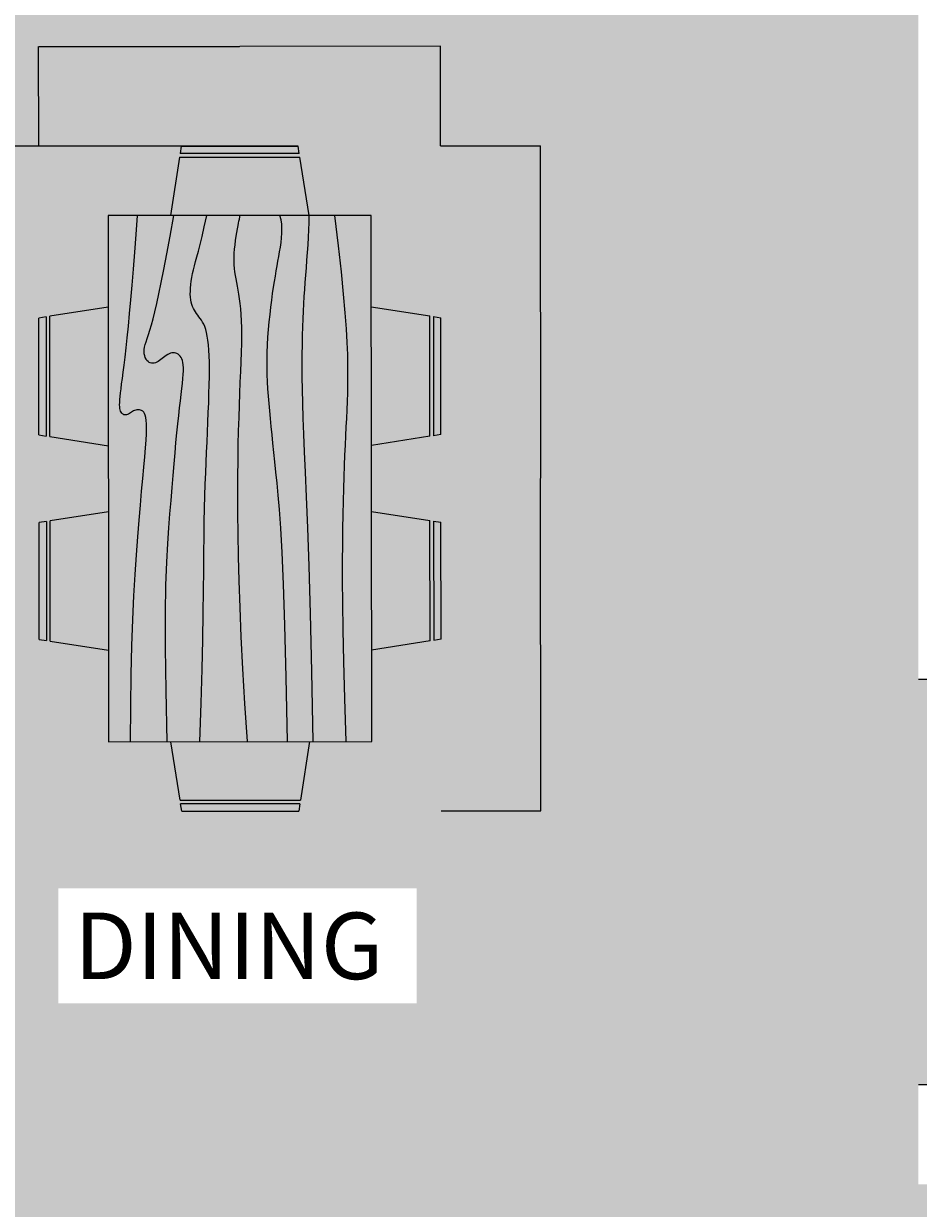
# Model space of a CAD drawing. Units: millimetres. Extents: x -229 to 16545, y -10488 to 4272.
# Tile 11 of 29: x 7347 to 9556, y -1268 to 1656. Entities that reach past the tile are written whole.
import ezdxf

# ---------------------------------------------------------------- set-up
doc = ezdxf.new("R2010")
doc.units = ezdxf.units.MM
for name, color, linetype, lineweight in [('A-ANNO-DIMS', 2, 'Continuous', 18), ('A-AREA-IDEN', 7, 'Continuous', 18), ('A-FURN', 8, 'Continuous', 18), ('A-FURN-PATT', 252, 'Continuous', 13)]:
    doc.layers.add(name, color=color, linetype=linetype, lineweight=lineweight)
doc.layers.add('A-FLOR-PATT', color=254, linetype='Continuous', lineweight=13, true_color=0xfeeab9)
doc.styles.get("Standard").update_dxf_attribs({"font": 'arial.ttf'})
doc.dimstyles.get("Standard").update_dxf_attribs({"dimtxt": 0.18, "dimasz": 0.18, "dimexe": 0.18, "dimexo": 0.0625, "dimgap": 0.09, "dimtad": 0, "dimtih": 1, "dimtoh": 1, "dimdec": 4, "dimzin": 0, "dimdsep": 46, "dimtxsty": 'Standard', "dimcen": 0.09, "dimadec": 0, "dimazin": 0, "dimtfac": 1, "dimtdec": 4, "dimtofl": 0, "dimtmove": 0, "dimatfit": 3, "dimfxl": 1, "dimtolj": 1, "dimtzin": 0, "dimarcsym": 0})

# ---------------------------------------------------------------- blocks, each defined once
blk = doc.blocks.new('Dining Set - 36 x 72 in.')
for p, q in [((-22.2343, 26.00059), (-23.4847, 17.99762)), ((-22.2304, 26), (-5.7608, 26)), ((-22, 27.5), (-22.1562, 26.50042)), ((-5.8416, 26.5), (-22.1534, 26.5)), ((-22, 27.5), (-6, 27.5)), ((-5.8437, 26.49966), (-6, 27.5)), ((-4.5152, 17.99762), (-5.7655, 25.99926)), ((5.7657, 26.00059), (4.5153, 17.99762)), ((5.7696, 26), (22.2392, 26)), ((6, 27.5), (5.8438, 26.50042)), ((22.1584, 26.5), (5.8466, 26.5)), ((6, 27.5), (22, 27.5)), ((22.1563, 26.49966), (22, 27.5)), ((23.4848, 17.99762), (22.2345, 25.99926)), ((36, 18), (-36, 18)), ((-36, 18), (-36, -18)), ((36, -18), (36, 18)), ((-45.5, 8), (-44.5004, 8.15617)), ((-44.5, -8.15843), (-44.5, 8.15338)), ((-44.0006, 8.23428), (-35.9976, 9.48474)), ((-44, 8.23041), (-44, -8.23915)), ((44.0006, 8.23428), (35.9976, 9.48474)), ((44, 8.23041), (44, -8.23915)), ((44.5, -8.15843), (44.5, 8.15338)), ((45.5, 8), (44.5005, 8.15617)), ((-45.5, 8), (-45.5, -8)), ((45.5, 8), (45.5, -8)), ((-44.4997, -8.15631), (-45.5, -8)), ((44.4997, -8.15631), (45.5, -8)), ((-35.9976, -9.48476), (-43.9993, -8.2345)), ((35.9976, -9.48476), (43.9993, -8.2345)), ((-36, -18), (36, -18)), ((-22.2343, -26.0006), (-23.4847, -17.99762)), ((-4.5152, -17.99762), (-5.7655, -25.99928)), ((5.7657, -26.0006), (4.5153, -17.99762)), ((23.4848, -17.99762), (22.2345, -25.99928)), ((-22.2304, -26), (-5.7608, -26)), ((-22, -27.5), (-22.1562, -26.50044)), ((-5.8416, -26.5), (-22.1534, -26.5)), ((-22, -27.5), (-6, -27.5)), ((-5.8437, -26.49967), (-6, -27.5)), ((5.7696, -26), (22.2392, -26)), ((6, -27.5), (5.8438, -26.50044)), ((22.1584, -26.5), (5.8466, -26.5)), ((6, -27.5), (22, -27.5)), ((22.1563, -26.49967), (22, -27.5))]:
    blk.add_line(p, q)
for points in [[(-36, 15), (-31.1772, 14.97754), (-26.8079, 14.91406), (-22.8538, 14.81543), (-19.276, 14.6875), (-16.0362, 14.53613), (-13.0957, 14.36718), (-10.4159, 14.18652), (-7.9583, 14), (-5.6904, 13.81315), (-3.6035, 13.63021), (-1.6954, 13.45508), (0.0365, 13.29166), (1.5945, 13.14388), (2.9811, 13.01562), (4.1988, 12.9108), (5.25, 12.83333), (6.1393, 12.78613), (6.8802, 12.76823), (7.4883, 12.77767), (7.9792, 12.8125), (8.3685, 12.87077), (8.6719, 12.95052), (8.9049, 13.0498), (9.0833, 13.16666), (9.2205, 13.29899), (9.3216, 13.44401), (9.3895, 13.59879), (9.4271, 13.76041), (9.4373, 13.92594), (9.4232, 14.09245), (9.3875, 14.257), (9.3333, 14.41666), (9.2638, 14.56917), (9.1836, 14.71484), (9.0975, 14.85465), (9.0104, 14.98958), (8.9272, 15.1206), (8.8529, 15.2487), (8.7922, 15.37483), (8.75, 15.5), (8.7305, 15.62467), (8.7344, 15.74739), (8.7617, 15.86621), (8.8125, 15.97916), (8.8867, 16.08431), (8.9844, 16.17968), (9.1055, 16.26334), (9.25, 16.33333), (9.4189, 16.38802), (9.6172, 16.42708), (9.8506, 16.45052), (10.125, 16.45833), (10.4463, 16.45052), (10.8203, 16.42708), (11.2529, 16.38802), (11.75, 16.33333), (12.3184, 16.26318), (12.9694, 16.17838), (13.7151, 16.07991), (14.5677, 15.96875), (15.5395, 15.84586), (16.6426, 15.71224), (17.8893, 15.56884), (19.2917, 15.41666), (20.859, 15.25667), (22.5879, 15.08984), (24.4721, 14.91715), (26.5052, 14.73958), (28.6809, 14.5581), (30.9929, 14.3737), (33.4347, 14.18733), (36, 14)], [(-36, 10), (-28.9766, 10.14274), (-23.1725, 10.20442), (-18.4241, 10.19775), (-14.5677, 10.13541), (-11.4399, 10.03011), (-8.877, 9.89453), (-6.7154, 9.74137), (-4.7917, 9.58333), (-2.9698, 9.43082), (-1.2246, 9.28515), (0.4415, 9.14534), (2.026, 9.01041), (3.5266, 8.87939), (4.9408, 8.7513), (6.266, 8.62516), (7.5, 8.5), (8.6411, 8.37549), (9.6914, 8.2539), (10.6538, 8.13818), (11.5312, 8.03125), (12.3267, 7.93603), (13.043, 7.85547), (13.6831, 7.79248), (14.25, 7.75), (14.7471, 7.7303), (15.1797, 7.73307), (15.5537, 7.75732), (15.875, 7.80208), (16.1494, 7.86637), (16.3828, 7.94922), (16.5811, 8.04964), (16.75, 8.16666), (16.8944, 8.29915), (17.0143, 8.44531), (17.1089, 8.60319), (17.1771, 8.77083), (17.218, 8.94629), (17.2305, 9.1276), (17.2137, 9.31282), (17.1667, 9.5), (17.0895, 9.6875), (16.987, 9.875), (16.8649, 10.0625), (16.7292, 10.25), (16.5856, 10.4375), (16.4401, 10.625), (16.2985, 10.8125), (16.1667, 11), (16.05, 11.18733), (15.9518, 11.3737), (15.8752, 11.5581), (15.8229, 11.73958), (15.798, 11.91715), (15.8034, 12.08984), (15.842, 12.25667), (15.9167, 12.41666), (16.0295, 12.56836), (16.1784, 12.70833), (16.3605, 12.83268), (16.5729, 12.9375), (16.8127, 13.01888), (17.0768, 13.07291), (17.3625, 13.0957), (17.6667, 13.08333), (17.9894, 13.03312), (18.3418, 12.94726), (18.7382, 12.82918), (19.1927, 12.68229), (19.7195, 12.51001), (20.3327, 12.31575), (21.0465, 12.10294), (21.875, 11.875), (22.8357, 11.63354), (23.959, 11.37304), (25.2786, 11.08618), (26.8282, 10.76562), (28.6414, 10.40405), (30.752, 9.99414), (33.1936, 9.52856), (36, 9)], [(-36, 5.5), (-30.7157, 5.3348), (-26.069, 5.20963), (-21.9946, 5.11767), (-18.4271, 5.05208), (-15.3009, 5.00602), (-12.5508, 4.97265), (-10.1112, 4.94515), (-7.9167, 4.91666), (-5.909, 4.88167), (-4.0586, 4.83984), (-2.3429, 4.79215), (-0.7396, 4.73958), (0.7739, 4.6831), (2.22, 4.6237), (3.6213, 4.56233), (5, 4.5), (6.373, 4.43782), (7.7344, 4.3776), (9.0723, 4.32129), (10.375, 4.27083), (11.6309, 4.22819), (12.8281, 4.19531), (13.9551, 4.17415), (15, 4.16666), (15.954, 4.17448), (16.819, 4.19791), (17.6001, 4.23698), (18.3021, 4.29166), (18.9299, 4.36198), (19.4883, 4.44791), (19.9823, 4.54948), (20.4167, 4.66666), (20.7969, 4.79899), (21.1302, 4.94401), (21.4245, 5.09879), (21.6875, 5.26041), (21.9271, 5.42594), (22.1511, 5.59245), (22.3672, 5.757), (22.5834, 5.91666), (22.8065, 6.06868), (23.0404, 6.21093), (23.2879, 6.34147), (23.5521, 6.45833), (23.8358, 6.55957), (24.142, 6.64323), (24.4735, 6.70735), (24.8334, 6.75), (25.2235, 6.76969), (25.642, 6.76692), (26.0858, 6.74267), (26.5521, 6.69791), (27.0379, 6.63362), (27.5404, 6.55078), (28.0565, 6.45036), (28.5834, 6.33333), (29.1242, 6.19987), (29.7071, 6.04687), (30.3661, 5.87044), (31.1354, 5.66666), (32.0493, 5.43164), (33.142, 5.16146), (34.4475, 4.85221), (36, 4.5)], [(-36, -1), (-30.7915, -0.6591), (-26.0195, -0.38216), (-21.6519, -0.16284), (-17.6563, 0.00521), (-14.0005, 0.12833), (-10.6523, 0.21289), (-7.5796, 0.26522), (-4.75, 0.29166), (-2.134, 0.29793), (0.2878, 0.28711), (2.5317, 0.26163), (4.6146, 0.22396), (6.5529, 0.17651), (8.3633, 0.12174), (10.0623, 0.06209), (11.6667, 0), (13.1899, -0.06201), (14.6341, -0.1211), (15.9982, -0.17432), (17.2813, -0.21875), (18.4823, -0.25147), (19.6003, -0.26953), (20.6343, -0.27002), (21.5834, -0.25), (22.4481, -0.20768), (23.2357, -0.14584), (23.9549, -0.06836), (24.6146, 0.02083), (25.2235, 0.11784), (25.7904, 0.21875), (26.3241, 0.31966), (26.8334, 0.41666), (27.3265, 0.50618), (27.8099, 0.58593), (28.2894, 0.65397), (28.7709, 0.70833), (29.2601, 0.74707), (29.763, 0.76823), (30.2855, 0.76985), (30.8334, 0.75), (31.4088, 0.70784), (31.9994, 0.64713), (32.589, 0.57275), (33.1615, 0.48958), (33.7008, 0.4025), (34.1908, 0.3164), (34.6153, 0.23616), (34.9584, 0.16666), (35.2099, 0.11165), (35.3848, 0.07031), (35.504, 0.04069), (35.5886, 0.02083), (35.6594, 0.00879), (35.7377, 0.0026), (35.8442, 0.00032), (36, 0)], [(-36, -6.5), (-27.1843, -6.31267), (-20.084, -6.1263), (-14.469, -5.9419), (-10.1094, -5.76042), (-6.7752, -5.58285), (-4.2363, -5.41016), (-2.2629, -5.24333), (-0.625, -5.08334), (0.8708, -4.93099), (2.2715, -4.78646), (3.5872, -4.64974), (4.8281, -4.52084), (6.0046, -4.39974), (7.127, -4.28646), (8.2053, -4.18099), (9.25, -4.08334), (10.2705, -3.99382), (11.2734, -3.91407), (12.2647, -3.84603), (13.25, -3.79167), (14.2354, -3.75293), (15.2266, -3.73177), (16.2295, -3.73015), (17.25, -3.75), (18.2912, -3.79248), (19.3451, -3.85547), (20.4009, -3.93604), (21.4479, -4.03125), (22.4754, -4.13819), (23.4727, -4.25391), (24.4289, -4.37549), (25.3334, -4.5), (26.1785, -4.62492), (26.9694, -4.74935), (27.7145, -4.87281), (28.4219, -4.99479), (29.1, -5.11483), (29.7572, -5.23242), (30.4016, -5.34709), (31.0417, -5.45834), (31.6837, -5.56437), (32.3262, -5.65821), (32.9658, -5.73153), (33.599, -5.77604), (34.2224, -5.78345), (34.8327, -5.74545), (35.4264, -5.65373), (36, -5.5)], [(-36, -10), (-26.4022, -9.81299), (-18.4675, -9.62891), (-11.9839, -9.45069), (-6.7396, -9.28125), (-2.5226, -9.12354), (0.8789, -8.98047), (3.6769, -8.85498), (6.0833, -8.75), (8.2767, -8.66765), (10.3021, -8.60677), (12.1712, -8.56543), (13.8958, -8.54167), (15.4876, -8.53353), (16.9583, -8.53907), (18.3197, -8.55632), (19.5834, -8.58334), (20.7616, -8.61841), (21.8685, -8.66081), (22.9188, -8.71004), (23.9271, -8.76563), (24.9081, -8.82707), (25.8763, -8.89388), (26.8465, -8.96558), (27.8334, -9.04167), (28.8474, -9.12118), (29.8828, -9.20117), (30.93, -9.27824), (31.9792, -9.34896), (33.0205, -9.40991), (34.0443, -9.45768), (35.0407, -9.48885), (36, -9.5)], [(-36, -14.5), (-30.0881, -14.33513), (-25.0332, -14.21224), (-20.7312, -14.12647), (-17.0781, -14.07292), (-13.97, -14.04671), (-11.3027, -14.04297), (-8.9724, -14.05681), (-6.875, -14.08334), (-4.9224, -14.11833), (-3.0905, -14.16016), (-1.3709, -14.20785), (0.2448, -14.26042), (1.7647, -14.3169), (3.1973, -14.3763), (4.5507, -14.43767), (5.8333, -14.5), (7.0554, -14.5621), (8.235, -14.62175), (9.3922, -14.67652), (10.5469, -14.72396), (11.7192, -14.76164), (12.929, -14.78711), (14.1965, -14.79794), (15.5417, -14.79167), (16.9933, -14.76424), (18.6152, -14.70508), (20.4804, -14.60197), (22.6615, -14.44271), (25.2312, -14.21509), (28.2624, -13.9069), (31.8277, -13.50594), (36, -13)]]:
    blk.add_lwpolyline(points)
blk = doc.blocks.new('*D35')
at = {"layer": 'A-ANNO-DIMS', "color": 0, "lineweight": -2, "transparency": 16777216}
for p, q in [((8376.7, 1354.7), (8623, 1354.9)), ((8622.8, 1354.7), (8623.5, 534.4)), ((8624.2, -286.3), (8623.5, 534)), ((8378.1, -286.6), (8624.4, -286.4))]:
    blk.add_line(p, q, dxfattribs=at)
at = {"layer": 'A-ANNO-DIMS', "color": 0, "transparency": 16777216}
for points in [[(8622.8, 1354.7), (8622.8, 1354.7), (8622.8, 1354.9)], [(8624.2, -286.3), (8624.2, -286.3), (8624.2, -286.4)]]:
    blk.add_solid(points, dxfattribs=at)
at = {"layer": 'Defpoints', "color": 0, "transparency": 16777216}
for p in [(8376.6, 1354.7), (8622.8, 1354.9), (8378, -286.6)]:
    blk.add_point(p, dxfattribs=at)
at = {"layer": 'A-ANNO-DIMS', "color": 0, "transparency": 16777216, "insert": (8623.5, 534.2), "char_height": 0.18, "attachment_point": 5}
blk.add_mtext('\\A1;DINING SET 1641', dxfattribs=at)
blk = doc.blocks.new('*D36')
at = {"layer": 'A-ANNO-DIMS', "color": 0, "lineweight": -2, "transparency": 16777216}
for p, q in [((7384.6, 1353.9), (7384.4, 1600.2)), ((7384.6, 1600), (7880.1, 1600.5)), ((8376.2, 1600.9), (7880.7, 1600.5)), ((8376.6, 1354.7), (8376.4, 1601.1))]:
    blk.add_line(p, q, dxfattribs=at)
at = {"layer": 'A-ANNO-DIMS', "color": 0, "transparency": 16777216}
for points in [[(7384.6, 1600.1), (7384.6, 1600), (7384.4, 1600)], [(8376.2, 1600.9), (8376.2, 1600.9), (8376.4, 1600.9)]]:
    blk.add_solid(points, dxfattribs=at)
at = {"layer": 'Defpoints', "color": 0, "transparency": 16777216}
for p in [(7384.4, 1600), (7384.6, 1353.8), (8376.6, 1354.7)]:
    blk.add_point(p, dxfattribs=at)
at = {"layer": 'A-ANNO-DIMS', "color": 0, "transparency": 16777216, "insert": (7880.4, 1600.5), "char_height": 0.18, "attachment_point": 5}
blk.add_mtext('\\A1;992', dxfattribs=at)
blk = doc.blocks.new('*D66')
at = {"layer": 'A-ANNO-DIMS', "color": 0, "lineweight": -2, "transparency": 16777216}
for p, q in [((9556, 38.2), (16544.5, 38.2)), ((16544.3, 38), (16544.3, -461.6)), ((16544.3, -961.6), (16544.3, -462)), ((9556, -961.8), (16544.5, -961.8))]:
    blk.add_line(p, q, dxfattribs=at)
at = {"layer": 'A-ANNO-DIMS', "color": 0, "transparency": 16777216}
for points in [[(16544.3, 38), (16544.4, 38), (16544.3, 38.2)], [(16544.3, -961.6), (16544.4, -961.6), (16544.3, -961.8)]]:
    blk.add_solid(points, dxfattribs=at)
at = {"layer": 'Defpoints', "color": 0, "transparency": 16777216}
for p in [(9555.9, 38.2), (9555.9, -961.8), (16544.3, -961.8)]:
    blk.add_point(p, dxfattribs=at)
at = {"layer": 'A-ANNO-DIMS', "color": 0, "transparency": 16777216, "insert": (16544.3, -461.8), "char_height": 0.18, "attachment_point": 5}
blk.add_mtext('\\A1;1000', dxfattribs=at)
blk = doc.blocks.new('*D100')
at = {"layer": 'A-ANNO-DIMS', "color": 0, "lineweight": -2, "transparency": 16777216}
for p, q in [((7294.4, 2021.7), (-228.8, 2021.7)), ((-228.7, 2021.5), (-228.7, 1688.2)), ((-228.7, 1354.6), (-228.7, 1687.9)), ((8024.8, 1354.4), (-228.8, 1354.4))]:
    blk.add_line(p, q, dxfattribs=at)
at = {"layer": 'A-ANNO-DIMS', "color": 0, "transparency": 16777216}
for points in [[(-228.7, 2021.5), (-228.6, 2021.5), (-228.7, 2021.7)], [(-228.7, 1354.6), (-228.6, 1354.6), (-228.7, 1354.4)]]:
    blk.add_solid(points, dxfattribs=at)
at = {"layer": 'Defpoints', "color": 0, "transparency": 16777216}
for p in [(7294.4, 2021.7), (-228.7, 1354.4), (8024.9, 1354.4)]:
    blk.add_point(p, dxfattribs=at)
at = {"layer": 'A-ANNO-DIMS', "color": 0, "transparency": 16777216, "insert": (-228.7, 1688.1), "char_height": 0.18, "attachment_point": 5}
blk.add_mtext('\\A1;667.3', dxfattribs=at)

msp = doc.modelspace()

# ---------------------------------------------------------------- hatches: boundary and pattern name
at = {"layer": 'A-FLOR-PATT', "transparency": 33554592}
h = msp.add_hatch(color=256, dxfattribs=at)
h.dxf.hatch_style = 1
h.paths.add_polyline_path([(7975.933, -5325.772), (7943.121, -5325.772), (7943.121, -4576.49, 0.40145271), (7225.933, -5325.772, 0.40145271), (6508.746, -4576.49), (6508.746, -5325.772), (6475.933, -5325.772), (6475.933, -5438.272), (5975.933, -5438.272), (5975.933, -7267.724), (5975.933, -7438.272), (6478.619, -7438.272), (6463.448, -7355.919), (6464.88, -7356.837), (6463.849, -7358.097), (6478.619, -7438.272), (6610.327, -7438.272), (6632.656, -7409.564), (6632.525, -7406.967), (6634.208, -7407.569), (6619.273, -7426.77), (6654.466, -7438.272), (7610.517, -7438.272), (7607.41, -7421.409), (7608.842, -7422.327), (7607.812, -7423.587), (7610.517, -7438.272), (7975.933, -7438.272)])
h.paths.add_polyline_path([(13785.933, -1208.272), (9555.933, -1208.272), (9555.933, -961.785), (9705.933, -961.785), (9705.933, -918.035), (10704.976, -918.035, 0.40145271), (9705.933, 38.215), (9555.933, 38.215), (9555.933, 2021.728), (5975.933, 2021.728), (5975.933, 755.492), (5745.933, 755.492), (5745.933, 1427.266), (2918.813, 1427.266), (2918.813, -492.942), (5013.319, -492.942), (5013.319, -978.272), (5745.933, -978.272), (5745.933, -397.513), (5975.933, -397.513), (5975.933, -1208.272), (4560.933, -1208.272), (4560.933, -1265.772), (4448.433, -1265.772), (4448.433, -1298.585), (4445.933, -1298.585), (3699.151, -1298.585, 0.40145271), (4448.433, -2015.772), (4560.933, -2015.772), (4560.933, -2384.177), (5745.933, -2384.177), (5799.402, -2384.177), (5799.402, -4518.272), (5975.933, -4518.272), (5975.933, -5208.272), (6475.933, -5208.272), (6475.933, -4575.772), (6508.746, -4575.772), (6508.746, -4576.49, -0.35647263), (7216.672, -5208.272), (7235.194, -5208.272, -0.35647263), (7943.121, -4576.49), (7943.121, -4575.772), (7975.933, -4575.772), (7975.933, -5208.272), (11176.247, -5208.272), (11159.44, -5191.465), (10520.768, -5191.465), (10520.768, -4888.936), (10571.19, -4888.936), (10571.19, -4872.129), (10772.876, -4872.129), (10772.876, -4888.936), (10789.683, -4888.936), (10789.683, -4872.129), (10991.368, -4872.129), (10991.368, -4888.936), (11041.79, -4888.936), (11041.79, -4872.129), (11058.597, -4872.129, -0.09090909), (11428.354, -4872.129), (11445.162, -4872.129), (11445.162, -4888.936), (11529.197, -4888.936), (11529.197, -5191.465), (11327.512, -5191.465), (11310.704, -5208.272), (13785.933, -5208.272)])
h.paths.add_polyline_path([(11047.216, -1630.944, -1), (11402.816, -1630.944, -1)], flags=16)
h.paths.add_polyline_path([(11148.816, -1630.944), (11225.016, -1554.744), (11301.216, -1630.944), (11225.016, -1707.144)], flags=0)
h.paths.add_polyline_path([(11199.616, -1630.944, -1), (11250.416, -1630.944, -1)], flags=0)
h.paths.add_polyline_path([(11588.751, -2096.259), (11588.751, -1543.254, -0.26666697), (12864.918, -1543.254), (12864.918, -2096.259), (12737.302, -2096.259), (12737.302, -2063.121), (11716.368, -2063.121), (11716.368, -2096.259)], flags=16)
h.paths.add_polyline_path([(12012.696, -2489.42), (12600.997, -2489.42), (12600.997, -3666.022), (12012.696, -3666.022)], flags=16)
h.paths.add_polyline_path([(12176.41, -3599.403), (12174.938, -3609.076), (12173.789, -3618.819), (12173.09, -3628.559), (12172.973, -3638.221), (12173.89, -3652.852), (12175.008, -3657.025), (12172.909, -3643.473), (12173.142, -3624.297), (12175.386, -3605.273)], flags=0)
h.paths.add_polyline_path([(8026.289, -286.944), (7737.703, -287.19), (7734.87, -269.156), (8029.092, -268.905)], flags=16)
h.paths.add_polyline_path([(7733.453, -260.139), (7710.784, -115.865), (7557.191, -115.996), (7556.999, 109.744), (7412.687, 132.166), (7412.433, 429.206), (7556.707, 451.876), (7556.568, 614.769), (7412.256, 637.19), (7412.003, 934.231), (7556.276, 956.9), (7556.084, 1182.639), (7709.677, 1182.77), (7732.099, 1327.082), (8029.14, 1327.335), (8051.808, 1183.062), (8205.401, 1183.192), (8205.594, 957.454), (8349.906, 935.031), (8350.159, 637.99), (8205.885, 615.322), (8206.024, 452.43), (8350.336, 430.006), (8350.59, 132.965), (8206.316, 110.298), (8206.509, -115.442), (8052.916, -115.573), (8030.493, -259.885)], flags=16)
h.paths.add_polyline_path([(12261.416, -3475.554), (12262.632, -3486.776), (12264.032, -3497.007), (12265.554, -3506.365), (12267.136, -3514.968), (12268.719, -3522.935), (12271.304, -3535.59), (12273.606, -3548.078), (12275.271, -3561.064), (12275.93, -3574.938), (12275.325, -3590.3), (12273.425, -3607.964), (12270.795, -3625.658), (12268.066, -3641.063), (12266.318, -3649.679), (12265.456, -3653.626), (12263.984, -3659.846), (12264.032, -3659.566), (12264.342, -3658.241), (12264.807, -3656.37), (12265.456, -3653.626), (12266.318, -3649.679), (12267.409, -3644.302), (12268.668, -3637.664), (12270.019, -3630.037), (12271.384, -3621.695), (12272.69, -3612.908), (12273.857, -3603.948), (12274.81, -3595.088), (12275.47, -3586.601), (12275.782, -3578.689), (12275.757, -3571.292), (12275.423, -3564.275), (12274.816, -3557.512), (12273.964, -3550.872), (12272.896, -3544.224), (12271.645, -3537.439), (12270.24, -3530.385), (12267.543, -3517.181), (12264.612, -3501.247), (12261.849, -3481.059)], flags=0)
h.paths.add_polyline_path([(12332.136, -3408.03), (12333.483, -3416.79), (12335.077, -3424.54), (12336.915, -3431.355), (12338.991, -3437.32), (12341.266, -3442.55), (12343.694, -3447.166), (12346.229, -3451.292), (12348.826, -3455.051), (12351.438, -3458.563), (12357.476, -3466.491), (12363.61, -3476.575), (12368.309, -3489.762), (12369.929, -3503.427), (12369.842, -3516.511), (12368.43, -3530.867), (12365.816, -3545.835), (12362.382, -3559.786), (12360.968, -3564.487), (12363.063, -3557.021), (12364.898, -3549.566), (12366.473, -3542.077), (12367.773, -3534.631), (12368.781, -3527.301), (12369.483, -3520.162), (12369.863, -3513.291), (12369.906, -3506.759), (12369.599, -3500.643), (12368.93, -3494.999), (12367.924, -3489.796), (12366.61, -3484.994), (12365.024, -3480.542), (12363.19, -3476.399), (12361.141, -3472.516), (12358.909, -3468.847), (12356.525, -3465.347), (12354.02, -3461.954), (12351.438, -3458.563), (12345.462, -3450.529), (12339.923, -3439.996), (12335.85, -3428.296), (12332.68, -3412.888)], flags=0)
h.paths.add_polyline_path([(12385.287, -3334.612), (12384.977, -3342.409), (12385.02, -3349.196), (12385.4, -3355.066), (12386.104, -3360.105), (12387.112, -3364.41), (12388.412, -3368.071), (12389.987, -3371.181), (12391.823, -3373.832), (12393.919, -3376.097), (12396.337, -3377.978), (12399.153, -3379.462), (12402.445, -3380.531), (12406.289, -3381.172), (12410.758, -3381.371), (12415.935, -3381.106), (12421.893, -3380.368), (12428.658, -3379.159), (12436.069, -3377.55), (12443.907, -3375.635), (12451.961, -3373.505), (12460.015, -3371.254), (12467.853, -3368.971), (12475.263, -3366.749), (12482.029, -3364.68), (12491.877, -3361.657), (12497.701, -3360.107), (12501.639, -3359.288), (12510.135, -3358.326), (12519.662, -3365.412), (12524.243, -3378.911), (12523.764, -3390.7), (12520.746, -3401.577), (12514.248, -3415.634), (12511.518, -3420.418), (12515.856, -3412.154), (12519.153, -3405.024), (12521.516, -3398.804), (12523.049, -3393.276), (12523.865, -3388.212), (12524.059, -3383.441), (12523.7, -3378.958), (12522.853, -3374.815), (12521.576, -3371.054), (12519.931, -3367.722), (12517.982, -3364.865), (12515.786, -3362.529), (12513.405, -3360.758), (12510.877, -3359.588), (12508.136, -3358.982), (12505.086, -3358.897), (12501.639, -3359.288), (12497.701, -3360.107), (12493.183, -3361.309), (12487.988, -3362.851), (12476.403, -3366.408), (12463.335, -3370.326), (12447.372, -3374.788), (12431.759, -3378.604), (12418.504, -3380.974), (12405.811, -3381.624), (12394.725, -3378.025), (12388.039, -3368.367), (12385.583, -3357.877), (12384.826, -3346.204), (12385.428, -3331.059), (12385.953, -3325.719)], flags=0)
h.paths.add_polyline_path([(7880.016, 1173.969), (7880.373, 1175.495), (7880.433, 1175.851), (7879.484, 1171.818)], flags=0)
h.paths.add_polyline_path([(7802.33, 874.962), (7800.771, 885.032), (7798.932, 893.941), (7796.811, 901.774), (7794.419, 908.63), (7791.798, 914.639), (7789.002, 919.945), (7786.083, 924.686), (7783.093, 929.005), (7780.087, 933.043), (7774.996, 939.717), (7768.406, 949.37), (7762.174, 963.427), (7759.342, 978.002), (7758.629, 991.888), (7759.492, 1007.928), (7761.801, 1025.496), (7765.392, 1044.035), (7766.625, 1049.048), (7764.522, 1039.543), (7762.719, 1030.232), (7761.232, 1021.168), (7760.08, 1012.405), (7759.28, 1003.994), (7758.849, 995.988), (7758.806, 988.44), (7759.167, 981.404), (7759.942, 974.914), (7761.104, 968.936), (7762.617, 963.414), (7764.448, 958.299), (7766.559, 953.535), (7768.918, 949.073), (7771.487, 944.856), (7774.232, 940.835), (7777.115, 936.938), (7782.377, 930.041), (7787.845, 922.139), (7793.348, 911.698), (7798.042, 898.247), (7801.702, 880.527)], flags=0)
h.paths.add_polyline_path([(12519.068, -3228.534), (12519.615, -3236.235), (12520.529, -3242.343), (12521.78, -3247.103), (12523.337, -3250.758), (12525.171, -3253.556), (12527.248, -3255.709), (12529.522, -3257.296), (12531.95, -3258.361), (12534.486, -3258.949), (12537.082, -3259.11), (12539.694, -3258.888), (12542.277, -3258.329), (12544.781, -3257.478), (12547.173, -3256.388), (12549.46, -3255.129), (12550.455, -3254.517), (12555.825, -3251.109), (12557.835, -3249.942), (12565.181, -3246.404), (12574.565, -3253.032), (12576.931, -3265.022), (12576.627, -3277.425), (12575.416, -3290.819), (12574.851, -3295.392), (12575.708, -3287.593), (12576.322, -3280.806), (12576.688, -3274.939), (12576.812, -3269.899), (12576.688, -3265.593), (12576.322, -3261.932), (12575.708, -3258.822), (12574.851, -3256.172), (12573.753, -3253.905), (12572.439, -3252.005), (12570.943, -3250.474), (12569.293, -3249.309), (12567.523, -3248.513), (12565.658, -3248.083), (12563.732, -3248.022), (12561.777, -3248.328), (12559.814, -3248.989), (12557.835, -3249.942), (12555.825, -3251.109), (12553.77, -3252.413), (12551.652, -3253.78), (12549.46, -3255.129), (12543.167, -3258.594), (12532.661, -3259.485), (12524.685, -3253.923), (12520.949, -3245.152), (12519.138, -3233.042)], flags=0)
h.paths.add_polyline_path([(7741.293, 790.501), (7741.641, 799.467), (7741.584, 807.269), (7741.141, 814.015), (7740.329, 819.809), (7739.165, 824.757), (7737.667, 828.966), (7735.853, 832.541), (7733.74, 835.586), (7731.348, 838.188), (7728.71, 840.348), (7725.861, 842.052), (7722.836, 843.28), (7719.671, 844.015), (7716.4, 844.237), (7713.06, 843.932), (7709.684, 843.081), (7706.304, 841.686), (7702.923, 839.834), (7699.543, 837.629), (7696.164, 835.178), (7692.784, 832.585), (7684.718, 826.315), (7675.609, 820.63), (7664.001, 817.274), (7654.105, 821.884), (7647.171, 832.02), (7644.191, 846.522), (7646.321, 860.288), (7647.49, 864.223), (7645.946, 857.865), (7645.046, 852.044), (7644.827, 846.557), (7645.243, 841.404), (7646.221, 836.642), (7647.693, 832.318), (7649.587, 828.489), (7651.832, 825.206), (7654.359, 822.523), (7657.097, 820.49), (7659.984, 819.145), (7662.993, 818.452), (7666.108, 818.357), (7669.311, 818.809), (7672.583, 819.755), (7675.908, 821.139), (7679.268, 822.913), (7682.645, 825.021), (7686.025, 827.401), (7689.404, 829.958), (7692.784, 832.585), (7700.505, 838.509), (7709.871, 843.64), (7721.436, 844.698), (7733.277, 837.617), (7739.571, 825.214), (7741.557, 811.049), (7741.669, 795.575)], flags=0)
h.paths.add_polyline_path([(8377.641, 137.216), (8359.607, 134.382), (8359.356, 428.605), (8377.395, 425.802)], flags=16)
h.paths.add_polyline_path([(7650.715, 668.465), (7650.08, 677.319), (7649.023, 684.34), (7647.579, 689.811), (7645.785, 694.012), (7643.675, 697.228), (7641.286, 699.7), (7638.669, 701.521), (7635.876, 702.744), (7632.96, 703.419), (7629.974, 703.601), (7626.971, 703.344), (7624.004, 702.697), (7621.125, 701.717), (7618.375, 700.462), (7615.749, 699.013), (7614.561, 698.279), (7608.435, 694.382), (7606.125, 693.04), (7598.981, 689.594), (7589.669, 693.773), (7585.26, 702.856), (7584.221, 713.11), (7584.49, 724.584), (7585.863, 739.937), (7586.518, 745.277), (7585.539, 736.31), (7584.841, 728.507), (7584.424, 721.761), (7584.288, 715.966), (7584.433, 711.016), (7584.86, 706.807), (7585.567, 703.231), (7586.556, 700.186), (7587.821, 697.58), (7589.332, 695.397), (7591.053, 693.637), (7592.951, 692.3), (7594.989, 691.385), (7597.132, 690.895), (7599.346, 690.826), (7601.594, 691.18), (7603.851, 691.943), (7606.125, 693.04), (7608.435, 694.382), (7610.797, 695.885), (7613.229, 697.458), (7620.475, 701.929), (7632.001, 704.44), (7643.476, 699.417), (7648.536, 687.571), (7650.63, 673.661)], flags=0)
h.paths.add_polyline_path([(7385.628, 136.37), (7385.382, 424.956), (7403.416, 427.789), (7403.667, 133.567)], flags=16)
h.paths.add_polyline_path([(12993.884, -2257.186), (12959.588, -2257.186), (12959.588, -2125.099), (13531.966, -2125.099, -0.19047621), (13531.966, -3974.321), (12959.588, -3974.321), (12959.588, -3842.233), (12993.884, -3842.233)], flags=16)
h.paths.add_polyline_path([(13413.486, -3313.884), (13413.486, -2785.535), (13562.885, -2785.535, -0.04962821), (13562.885, -3313.884)], flags=0)
h.paths.add_polyline_path([(8377.21, 642.241), (8359.176, 639.407), (8358.925, 933.629), (8376.964, 930.826)], flags=16)
h.paths.add_polyline_path([(13086.058, -1864.83), (13086.058, -1449.84), (13501.048, -1449.84), (13501.048, -1864.83)], flags=16)
h.paths.add_polyline_path([(13305.814, -1862.197), (13302.103, -1859.624), (13298.088, -1857.068), (13293.799, -1854.536), (13289.262, -1852.031), (13284.504, -1849.559), (13279.554, -1847.125), (13274.439, -1844.735), (13269.17, -1842.389), (13263.701, -1840.081), (13257.97, -1837.797), (13251.914, -1835.525), (13245.472, -1833.252), (13238.582, -1830.968), (13231.18, -1828.66), (13223.206, -1826.315), (13209.182, -1822.458), (13204.584, -1821.48), (13217.962, -1824.773), (13235.072, -1829.804), (13248.777, -1834.349), (13260.829, -1838.869), (13274.479, -1844.63), (13289.675, -1852.101), (13302.553, -1859.704)], flags=0)
h.paths.add_polyline_path([(13428.104, -1820.994), (13419.007, -1818.141), (13409.95, -1815.4), (13400.766, -1812.747), (13391.271, -1810.151), (13376.087, -1806.251), (13370.618, -1805.019), (13386.304, -1808.794), (13405.087, -1813.928), (13423.014, -1819.354)], flags=0)
h.paths.add_polyline_path([(7385.197, 641.395), (7384.951, 929.98), (7402.986, 932.814), (7403.236, 638.592)], flags=16)
h.paths.add_polyline_path([(13262.537, -1725.526), (13253.246, -1724.74), (13244.516, -1724.117), (13235.94, -1723.625), (13223.267, -1723.062), (13217.598, -1722.912), (13231.966, -1723.397), (13248.733, -1724.359), (13266.899, -1725.895), (13272.802, -1726.502)], flags=0)
h.paths.add_polyline_path([(13191.893, -1641.137), (13208.675, -1640.506), (13214.057, -1640.258), (13197.763, -1640.936)], flags=0)
h.paths.add_polyline_path([(13097.524, -1608.457), (13114.284, -1609.031), (13120.126, -1609.105), (13103.045, -1608.71)], flags=0)
h.paths.add_polyline_path([(13465.328, -1521.577), (13473.906, -1517.015), (13481.761, -1511.636), (13492.562, -1502.076), (13495.327, -1497.933), (13485.818, -1508.858), (13470.208, -1519.547)], flags=0)
h.paths.add_polyline_path([(13175.015, -1500.891), (13184.046, -1501.807), (13192.721, -1502.52), (13201.114, -1503.034), (13209.273, -1503.351), (13217.244, -1503.476), (13225.078, -1503.41), (13232.821, -1503.16), (13240.524, -1502.728), (13248.233, -1502.117), (13255.993, -1501.322), (13263.825, -1500.293), (13271.746, -1498.974), (13279.775, -1497.305), (13287.928, -1495.229), (13296.222, -1492.688), (13304.675, -1489.622), (13313.304, -1485.975), (13322.089, -1481.727), (13330.859, -1477.028), (13339.408, -1472.063), (13347.526, -1467.02), (13355.006, -1462.087), (13364.86, -1455.202), (13367.224, -1453.299), (13358.544, -1459.754), (13343.348, -1469.775), (13326.143, -1479.767), (13309.023, -1488.045), (13292.249, -1494.129), (13276.009, -1498.264), (13260.299, -1500.88), (13244.401, -1502.51), (13228.945, -1503.378), (13213.316, -1503.508), (13197.047, -1502.876), (13180.088, -1501.481)], flags=0)
h.paths.add_polyline_path([(7733.501, 1336.101), (7736.303, 1354.14), (8024.889, 1354.386), (8027.723, 1336.352)], flags=16)
at = {"layer": 'A-FURN-PATT', "transparency": 33554569}
h = msp.add_hatch(color=256, dxfattribs=at)
h.dxf.hatch_style = 1
h.paths.add_polyline_path([(8029.14, 1327.335), (7732.099, 1327.082), (7709.677, 1182.77), (8051.808, 1183.062)])
h.paths.add_polyline_path([(8024.889, 1354.386), (7736.303, 1354.14), (7733.501, 1336.101), (8027.723, 1336.352)])
h.paths.add_polyline_path([(8349.906, 935.031), (8205.594, 957.454), (8205.885, 615.322), (8350.159, 637.99)])
h.paths.add_polyline_path([(8376.964, 930.826), (8358.925, 933.629), (8359.176, 639.407), (8377.21, 642.241)])
h.paths.add_polyline_path([(8350.336, 430.006), (8206.024, 452.43), (8206.316, 110.298), (8350.59, 132.965)])
h.paths.add_polyline_path([(8377.395, 425.802), (8359.356, 428.605), (8359.607, 134.382), (8377.641, 137.216)])
h.paths.add_polyline_path([(8052.916, -115.573), (7710.784, -115.865), (7733.453, -260.139), (8030.493, -259.885)])
h.paths.add_polyline_path([(8029.092, -268.905), (7734.87, -269.156), (7737.703, -287.19), (8026.289, -286.944)])
h.paths.add_polyline_path([(7556.707, 451.876), (7412.433, 429.206), (7412.687, 132.166), (7556.999, 109.744)])
h.paths.add_polyline_path([(7403.416, 427.789), (7385.382, 424.956), (7385.628, 136.37), (7403.667, 133.567)])
h.paths.add_polyline_path([(7556.276, 956.9), (7412.003, 934.231), (7412.256, 637.19), (7556.568, 614.769)])
h = msp.add_hatch(color=256, dxfattribs=at)
h.dxf.hatch_style = 1
h.paths.add_polyline_path([(7883.255, 797.549), (7884.194, 822.154), (7884.976, 845.297), (7885.547, 866.96), (7885.856, 887.125), (7885.849, 905.775), (7885.473, 922.893), (7884.697, 938.489), (7883.569, 952.693), (7882.161, 965.664), (7880.542, 977.561), (7878.783, 988.542), (7876.954, 998.766), (7875.126, 1008.39), (7873.368, 1017.575), (7871.746, 1026.467), (7870.3, 1035.185), (7869.066, 1043.833), (7868.078, 1052.516), (7867.371, 1061.339), (7866.982, 1070.41), (7866.945, 1079.834), (7867.294, 1089.716), (7868.046, 1100.095), (7869.132, 1110.748), (7870.464, 1121.384), (7871.956, 1131.711), (7873.518, 1141.44), (7875.063, 1150.279), (7876.504, 1157.937), (7877.752, 1164.126), (7879.021, 1169.949), (7880.016, 1173.969), (7880.373, 1175.495), (7880.589, 1176.772), (7880.699, 1178.185), (7880.739, 1180.106), (7880.742, 1182.916), (7799.578, 1182.846), (7793.249, 1154.839), (7787.691, 1131.288), (7782.835, 1111.575), (7778.61, 1095.088), (7774.946, 1081.209), (7771.774, 1069.32), (7769.024, 1058.804), (7766.625, 1049.048), (7764.522, 1039.543), (7762.719, 1030.232), (7761.232, 1021.168), (7760.08, 1012.405), (7759.28, 1003.994), (7758.849, 995.988), (7758.806, 988.44), (7759.167, 981.404), (7759.942, 974.914), (7761.104, 968.936), (7762.617, 963.414), (7764.448, 958.299), (7766.559, 953.535), (7768.918, 949.073), (7771.487, 944.856), (7774.232, 940.835), (7777.115, 936.938), (7782.377, 930.041), (7786.083, 924.686), (7789.002, 919.945), (7791.798, 914.639), (7794.419, 908.63), (7796.811, 901.774), (7798.932, 893.941), (7800.771, 885.032), (7802.33, 874.962), (7803.608, 863.64), (7804.605, 850.979), (7805.321, 836.891), (7805.757, 821.29), (7805.913, 804.083), (7805.794, 785.237), (7805.43, 764.909), (7804.855, 743.315), (7804.105, 720.662), (7803.215, 697.165), (7802.22, 673.033), (7801.155, 648.477), (7800.055, 623.712), (7798.952, 598.844), (7797.866, 573.568), (7796.817, 547.485), (7795.822, 520.185), (7794.898, 491.267), (7794.064, 460.32), (7793.338, 426.945), (7792.738, 390.732), (7792.258, 351.151), (7791.799, 307.148), (7791.24, 257.545), (7790.457, 201.158), (7789.329, 136.812), (7787.733, 63.322), (7785.547, -20.49), (7782.649, -115.804), (7899.886, -115.704), (7893.658, -21.765), (7888.589, 64.301), (7884.566, 143.074), (7881.474, 215.139), (7879.197, 281.075), (7877.62, 341.464), (7876.629, 396.884), (7876.109, 447.92), (7875.955, 495.104), (7876.113, 538.785), (7876.538, 579.257), (7877.186, 616.826), (7878.012, 651.788), (7878.972, 684.442), (7880.021, 715.087), (7881.117, 744.026), (7882.212, 771.5)])
h.paths.add_polyline_path([(7948.326, 826.381), (7948.668, 844.787), (7949.418, 863.568), (7950.538, 882.577), (7951.975, 901.622), (7953.676, 920.507), (7955.589, 939.042), (7957.661, 957.031), (7959.839, 974.28), (7962.071, 990.596), (7964.311, 1005.84), (7966.543, 1020.107), (7968.759, 1033.548), (7970.948, 1046.309), (7973.103, 1058.542), (7975.213, 1070.397), (7977.272, 1082.022), (7979.268, 1093.569), (7981.171, 1105.15), (7982.854, 1116.74), (7984.166, 1128.277), (7984.959, 1139.699), (7985.083, 1150.943), (7984.389, 1161.95), (7982.725, 1172.657), (7979.944, 1183), (7880.742, 1182.916), (7880.735, 1177.044), (7880.016, 1173.969), (7879.484, 1171.818), (7878.741, 1168.663), (7877.752, 1164.126), (7876.504, 1157.937), (7875.063, 1150.279), (7873.518, 1141.44), (7871.956, 1131.711), (7870.464, 1121.384), (7869.132, 1110.748), (7868.046, 1100.095), (7867.294, 1089.716), (7866.945, 1079.834), (7866.982, 1070.41), (7867.371, 1061.339), (7868.078, 1052.516), (7869.066, 1043.833), (7870.3, 1035.185), (7871.746, 1026.467), (7873.368, 1017.575), (7875.126, 1008.39), (7876.954, 998.766), (7878.783, 988.542), (7880.542, 977.561), (7882.161, 965.664), (7883.569, 952.693), (7884.697, 938.489), (7885.473, 922.893), (7885.849, 905.775), (7885.856, 887.125), (7885.547, 866.96), (7884.976, 845.297), (7884.194, 822.154), (7883.255, 797.549), (7882.212, 771.5), (7881.117, 744.026), (7880.021, 715.087), (7878.972, 684.442), (7878.012, 651.788), (7877.186, 616.826), (7876.538, 579.257), (7876.113, 538.785), (7875.955, 495.104), (7876.109, 447.92), (7876.629, 396.884), (7877.62, 341.464), (7879.197, 281.075), (7881.474, 215.139), (7884.566, 143.074), (7888.589, 64.301), (7893.658, -21.765), (7899.886, -115.704), (7999.088, -115.619), (7995.573, 43.383), (7992.103, 171.446), (7988.69, 272.718), (7985.35, 351.348), (7982.096, 411.483), (7978.942, 457.273), (7975.903, 492.864), (7972.992, 522.404), (7970.221, 549.38), (7967.593, 574.642), (7965.106, 598.371), (7962.762, 620.75), (7960.56, 641.968), (7958.5, 662.211), (7956.581, 681.658), (7954.803, 700.5), (7953.173, 718.905), (7951.719, 736.992), (7950.477, 754.871), (7949.481, 772.641), (7948.767, 790.414), (7948.37, 808.292)])
h.paths.add_polyline_path([(8035.051, 839.6), (8035.341, 864.155), (8035.809, 886.948), (8036.424, 908.199), (8037.171, 928.165), (8038.043, 947.109), (8039.03, 965.296), (8040.123, 982.991), (8041.313, 1000.455), (8042.592, 1017.956), (8043.949, 1035.757), (8045.367, 1054.047), (8046.794, 1072.724), (8048.168, 1091.613), (8049.428, 1110.538), (8050.511, 1129.32), (8051.357, 1147.787), (8051.904, 1165.759), (8052.072, 1181.384), (8051.808, 1183.062), (7979.944, 1183), (7982.725, 1172.657), (7984.389, 1161.95), (7985.083, 1150.943), (7984.959, 1139.699), (7984.166, 1128.277), (7982.854, 1116.74), (7981.171, 1105.15), (7979.268, 1093.569), (7977.272, 1082.022), (7975.213, 1070.397), (7973.103, 1058.542), (7970.948, 1046.309), (7968.759, 1033.548), (7966.543, 1020.107), (7964.311, 1005.84), (7962.071, 990.596), (7959.839, 974.28), (7957.661, 957.031), (7955.589, 939.042), (7953.676, 920.507), (7951.975, 901.622), (7950.538, 882.577), (7949.418, 863.568), (7948.668, 844.787), (7948.326, 826.381), (7948.37, 808.292), (7948.767, 790.414), (7949.481, 772.641), (7950.477, 754.871), (7951.719, 736.992), (7953.173, 718.905), (7954.803, 700.5), (7956.581, 681.658), (7958.5, 662.211), (7960.56, 641.968), (7962.762, 620.75), (7965.106, 598.371), (7967.593, 574.642), (7970.221, 549.38), (7972.992, 522.404), (7975.903, 492.864), (7978.942, 457.273), (7982.096, 411.483), (7985.35, 351.348), (7988.69, 272.718), (7992.103, 171.446), (7995.573, 43.383), (7999.088, -115.619), (8062.216, -115.565), (8058.695, 57.543), (8055.253, 200.656), (8051.939, 317.595), (8048.802, 412.182), (8045.892, 488.239), (8043.26, 549.589), (8040.953, 600.053), (8039.023, 643.455), (8037.504, 683.015), (8036.374, 719.545), (8035.6, 753.257), (8035.145, 784.363), (8034.974, 813.073)])
h.paths.add_polyline_path([(8146.239, 869.579), (8144.351, 903.22), (8141.445, 942.557), (8137.3, 988.902), (8131.694, 1043.57), (8124.408, 1107.869), (8115.218, 1183.116), (8052.09, 1183.062), (8051.904, 1165.759), (8051.357, 1147.787), (8050.511, 1129.32), (8049.428, 1110.538), (8048.168, 1091.613), (8046.794, 1072.724), (8045.367, 1054.047), (8043.949, 1035.757), (8042.592, 1017.956), (8041.313, 1000.455), (8040.123, 982.991), (8039.03, 965.296), (8038.043, 947.109), (8037.171, 928.165), (8036.424, 908.199), (8035.809, 886.948), (8035.341, 864.155), (8035.051, 839.6), (8034.974, 813.073), (8035.145, 784.363), (8035.6, 753.257), (8036.374, 719.545), (8037.504, 683.015), (8039.023, 643.455), (8040.953, 600.053), (8043.26, 549.589), (8045.892, 488.239), (8048.802, 412.182), (8051.939, 317.595), (8055.253, 200.656), (8058.695, 57.543), (8062.216, -115.565), (8143.38, -115.496), (8140.316, -8.868), (8138.022, 82.303), (8136.408, 159.895), (8135.386, 225.784), (8134.866, 281.843), (8134.757, 329.952), (8134.971, 371.983), (8135.417, 409.813), (8136.018, 445.032), (8136.745, 478.074), (8137.578, 509.09), (8138.502, 538.233), (8139.497, 565.648), (8140.546, 591.488), (8141.632, 615.899), (8142.737, 639.034), (8143.838, 661.078), (8144.896, 682.355), (8145.866, 703.227), (8146.704, 724.055), (8147.366, 745.2), (8147.806, 767.021), (8147.982, 789.882), (8147.848, 814.145), (8147.331, 840.327)])
h.paths.add_polyline_path([(8205.401, 1183.192), (8115.218, 1183.116), (8124.408, 1107.869), (8131.694, 1043.57), (8137.3, 988.902), (8141.445, 942.557), (8144.351, 903.22), (8146.239, 869.579), (8147.331, 840.327), (8147.848, 814.145), (8147.982, 789.882), (8147.806, 767.021), (8147.366, 745.2), (8146.704, 724.055), (8145.866, 703.227), (8144.896, 682.355), (8143.838, 661.078), (8142.737, 639.034), (8141.632, 615.899), (8140.546, 591.488), (8139.497, 565.648), (8138.502, 538.233), (8137.578, 509.09), (8136.745, 478.074), (8136.018, 445.032), (8135.417, 409.813), (8134.971, 371.983), (8134.757, 329.952), (8134.866, 281.843), (8135.386, 225.784), (8136.408, 159.895), (8138.022, 82.303), (8140.316, -8.868), (8143.38, -115.496), (8206.509, -115.442)])
h.paths.add_polyline_path([(7741.293, 790.501), (7741.641, 799.467), (7741.584, 807.269), (7741.141, 814.015), (7740.329, 819.809), (7739.165, 824.757), (7737.667, 828.966), (7735.853, 832.541), (7733.74, 835.586), (7731.348, 838.188), (7728.71, 840.348), (7725.861, 842.052), (7722.836, 843.28), (7719.671, 844.015), (7716.4, 844.237), (7713.06, 843.932), (7709.684, 843.081), (7706.304, 841.686), (7702.923, 839.834), (7699.543, 837.629), (7696.164, 835.178), (7692.784, 832.585), (7686.987, 828.079), (7680.802, 823.724), (7674.136, 820.204), (7667.592, 818.312), (7661.367, 818.501), (7655.629, 821.174), (7650.522, 826.598), (7647.693, 832.318), (7646.221, 836.642), (7645.243, 841.404), (7644.827, 846.557), (7645.046, 852.044), (7645.946, 857.865), (7647.49, 864.223), (7649.613, 871.374), (7652.256, 879.574), (7655.355, 889.078), (7658.849, 900.141), (7662.677, 913.019), (7666.775, 927.966), (7671.115, 945.298), (7675.797, 965.562), (7680.95, 989.368), (7686.708, 1017.322), (7693.202, 1050.032), (7700.563, 1088.106), (7708.923, 1132.151), (7718.413, 1182.777), (7628.23, 1182.7), (7624.891, 1136.428), (7621.567, 1092.383), (7618.276, 1050.68), (7615.037, 1011.435), (7611.865, 974.762), (7608.779, 940.775), (7605.797, 909.589), (7602.935, 881.318), (7600.212, 856.021), (7597.645, 833.532), (7595.252, 813.634), (7593.05, 796.104), (7591.058, 780.725), (7589.294, 767.273), (7587.774, 755.53), (7586.518, 745.277), (7585.539, 736.31), (7584.841, 728.507), (7584.424, 721.761), (7584.288, 715.966), (7584.433, 711.016), (7584.86, 706.807), (7585.567, 703.231), (7586.556, 700.186), (7587.821, 697.58), (7589.332, 695.397), (7591.053, 693.637), (7592.951, 692.3), (7594.989, 691.385), (7597.132, 690.895), (7599.346, 690.826), (7601.594, 691.18), (7603.851, 691.943), (7606.125, 693.04), (7608.435, 694.382), (7610.797, 695.885), (7616.667, 699.681), (7622.602, 702.392), (7628.548, 703.687), (7634.553, 703.323), (7640.155, 700.871), (7644.996, 695.86), (7647.579, 689.811), (7649.023, 684.34), (7650.08, 677.319), (7650.715, 668.465), (7650.895, 657.497), (7650.583, 644.134), (7649.746, 628.093), (7648.365, 609.132), (7646.493, 587.167), (7644.201, 562.155), (7641.559, 534.052), (7638.638, 502.812), (7635.509, 468.394), (7632.241, 430.75), (7628.906, 389.842), (7625.58, 345.513), (7622.363, 297.175), (7619.361, 244.136), (7616.68, 185.699), (7614.428, 121.166), (7612.71, 49.846), (7611.632, -28.963), (7611.301, -115.95), (7701.484, -115.873), (7698.801, 10.803), (7697.6, 115.488), (7697.647, 201.133), (7698.712, 270.691), (7700.563, 327.107), (7702.969, 373.335), (7705.698, 412.325), (7708.519, 447.025), (7711.242, 479.888), (7713.842, 511.368), (7716.339, 541.421), (7718.748, 570.002), (7721.088, 597.07), (7723.376, 622.579), (7725.631, 646.483), (7727.87, 668.742), (7730.098, 689.325), (7732.275, 708.271), (7734.347, 725.631), (7736.262, 741.458), (7737.968, 755.808), (7739.41, 768.729), (7740.536, 780.275)])
h.paths.add_polyline_path([(7802.33, 874.962), (7800.771, 885.032), (7798.932, 893.941), (7796.811, 901.774), (7794.419, 908.63), (7791.798, 914.639), (7789.002, 919.945), (7786.083, 924.686), (7783.093, 929.005), (7780.087, 933.043), (7774.996, 939.717), (7771.487, 944.856), (7768.918, 949.073), (7766.559, 953.535), (7764.448, 958.299), (7762.617, 963.414), (7761.104, 968.936), (7759.942, 974.914), (7759.167, 981.404), (7758.806, 988.44), (7758.849, 995.988), (7759.28, 1003.994), (7760.08, 1012.405), (7761.232, 1021.168), (7762.719, 1030.232), (7764.522, 1039.543), (7766.625, 1049.048), (7769.024, 1058.804), (7771.774, 1069.32), (7774.946, 1081.209), (7778.61, 1095.088), (7782.835, 1111.575), (7787.691, 1131.288), (7793.249, 1154.839), (7799.578, 1182.846), (7718.413, 1182.777), (7708.923, 1132.151), (7700.563, 1088.106), (7693.202, 1050.032), (7686.708, 1017.322), (7680.95, 989.368), (7675.797, 965.562), (7671.115, 945.298), (7666.775, 927.966), (7662.677, 913.019), (7658.849, 900.141), (7655.355, 889.078), (7652.256, 879.574), (7649.613, 871.374), (7647.49, 864.223), (7645.946, 857.865), (7645.046, 852.044), (7644.827, 846.557), (7645.243, 841.404), (7646.221, 836.642), (7647.693, 832.318), (7649.587, 828.489), (7651.832, 825.206), (7654.359, 822.523), (7657.097, 820.49), (7659.984, 819.145), (7662.993, 818.452), (7666.108, 818.357), (7669.311, 818.809), (7672.583, 819.755), (7675.908, 821.139), (7679.268, 822.913), (7682.645, 825.021), (7686.025, 827.401), (7689.404, 829.958), (7695.508, 834.703), (7701.539, 839.075), (7708.141, 842.692), (7714.726, 844.351), (7721.298, 843.904), (7727.384, 841.434), (7732.705, 837.077), (7736.965, 830.939), (7739.165, 824.757), (7740.329, 819.809), (7741.141, 814.015), (7741.584, 807.269), (7741.641, 799.467), (7741.293, 790.501), (7740.536, 780.275), (7739.41, 768.729), (7737.968, 755.808), (7736.262, 741.458), (7734.347, 725.631), (7732.275, 708.271), (7730.098, 689.325), (7727.87, 668.742), (7725.631, 646.483), (7723.376, 622.579), (7721.088, 597.07), (7718.748, 570.002), (7716.339, 541.421), (7713.842, 511.368), (7711.242, 479.888), (7708.519, 447.025), (7705.698, 412.325), (7702.969, 373.335), (7700.563, 327.107), (7698.712, 270.691), (7697.647, 201.133), (7697.6, 115.488), (7698.801, 10.803), (7701.484, -115.873), (7782.649, -115.804), (7785.547, -20.49), (7787.733, 63.322), (7789.329, 136.812), (7790.457, 201.158), (7791.24, 257.545), (7791.799, 307.148), (7792.258, 351.151), (7792.738, 390.732), (7793.338, 426.945), (7794.064, 460.32), (7794.898, 491.267), (7795.822, 520.185), (7796.817, 547.485), (7797.866, 573.568), (7798.952, 598.844), (7800.055, 623.712), (7801.155, 648.477), (7802.22, 673.033), (7803.215, 697.165), (7804.105, 720.662), (7804.855, 743.315), (7805.43, 764.909), (7805.794, 785.237), (7805.913, 804.083), (7805.757, 821.29), (7805.321, 836.891), (7804.605, 850.979), (7803.608, 863.64)])
h.paths.add_polyline_path([(7647.579, 689.811), (7645.785, 694.012), (7643.675, 697.228), (7641.286, 699.7), (7638.669, 701.521), (7635.876, 702.744), (7632.96, 703.419), (7629.974, 703.601), (7626.971, 703.344), (7624.004, 702.697), (7621.125, 701.717), (7618.375, 700.462), (7615.749, 699.013), (7613.229, 697.458), (7607.197, 693.557), (7601.404, 690.763), (7596.004, 690.93), (7591.899, 692.772), (7588.436, 696.314), (7585.904, 701.529), (7584.86, 706.807), (7584.433, 711.016), (7584.288, 715.966), (7584.424, 721.761), (7584.841, 728.507), (7585.539, 736.31), (7586.518, 745.277), (7587.774, 755.53), (7589.294, 767.273), (7591.058, 780.725), (7593.05, 796.104), (7595.252, 813.634), (7597.645, 833.532), (7600.212, 856.021), (7602.935, 881.318), (7605.797, 909.589), (7608.779, 940.775), (7611.865, 974.762), (7615.037, 1011.435), (7618.276, 1050.68), (7621.567, 1092.383), (7624.891, 1136.428), (7628.23, 1182.7), (7556.084, 1182.639), (7557.191, -115.996), (7611.301, -115.95), (7611.632, -28.963), (7612.71, 49.846), (7614.428, 121.166), (7616.68, 185.699), (7619.361, 244.136), (7622.363, 297.175), (7625.58, 345.513), (7628.906, 389.842), (7632.241, 430.75), (7635.509, 468.394), (7638.638, 502.812), (7641.559, 534.052), (7644.201, 562.155), (7646.493, 587.167), (7648.365, 609.132), (7649.746, 628.093), (7650.583, 644.134), (7650.895, 657.497), (7650.715, 668.465), (7650.08, 677.319), (7649.023, 684.34)])
at = {"layer": 'A-FURN-PATT'}
h = msp.add_hatch(color=256, dxfattribs=at)
h.dxf.hatch_style = 1
h.paths.add_polyline_path([(7402.986, 932.814), (7384.951, 929.98), (7385.197, 641.395), (7403.236, 638.592)])

# ---------------------------------------------------------------- block references
at = {"layer": 'A-FURN', "xscale": 18.03659995736163, "yscale": 18.03659995736163, "zscale": 18.03659995736163, "rotation": 90.04886308873441}
msp.add_blockref('Dining Set - 36 x 72 in.', (7881.296, 533.598), dxfattribs=at)

# ---------------------------------------------------------------- dimensions: what is measured, and where the dimension line sits
at = {"layer": 'A-ANNO-DIMS'}
for base, p1, p2, angle, override, picture, middle in [((-228.657, 1354.386), (7294.425, 2021.728), (8024.889, 1354.386), 90, {"dimdec": 1, "dimlfac": 1, "dimrnd": 0, "dimzin": 0, "dimdsep": 46, "dimlunit": 2}, '*D100', (-228.657, 1688.057)), ((7384.38, 1600.04), (8376.603, 1354.686), (7384.59, 1353.84), 180.048863, {"dimdec": 0, "dimlfac": 1, "dimrnd": 0, "dimzin": 0, "dimdsep": 46, "dimlunit": 2}, '*D36', (7880.386, 1600.463)), ((16544.342, -961.785), (9555.933, 38.215), (9555.933, -961.785), 90, {"dimdec": 0, "dimlfac": 1, "dimrnd": 0, "dimzin": 0, "dimdsep": 46, "dimlunit": 2}, '*D66', (16544.342, -461.785))]:
    dim = msp.add_linear_dim(base=base, p1=p1, p2=p2, angle=angle, dimstyle='Standard', override=override, dxfattribs=at)
    dim.commit()
    dim.dimension.update_dxf_attribs({"geometry": picture, "text_midpoint": middle})
dim = msp.add_linear_dim(base=(8622.802, 1354.896), p1=(8378.002, -286.644), p2=(8376.603, 1354.686), angle=90.048863, text='DINING SET <>', dimstyle='Standard', override={"dimdec": 0, "dimlfac": 1, "dimrnd": 0, "dimzin": 0, "dimdsep": 46, "dimlunit": 2}, dxfattribs=at)
dim.commit()
dim.dimension.update_dxf_attribs({"geometry": '*D35', "text_midpoint": (8623.502, 534.231)})

# ---------------------------------------------------------------- next in the draw order: wipeouts: each hides what was drawn before it
msp.add_wipeout([(7432.587, -762.019), (8317.502, -762.019), (8317.502, -477.551), (7432.587, -477.551)]).dxf.layer = 'A-AREA-IDEN'

# ---------------------------------------------------------------- next in the draw order: texts
at = {"layer": 'A-AREA-IDEN'}
msp.add_text('DINING', height=164.0431, dxfattribs=at).set_placement((7472.322, -701.806))

doc.saveas('drawing.dxf')
